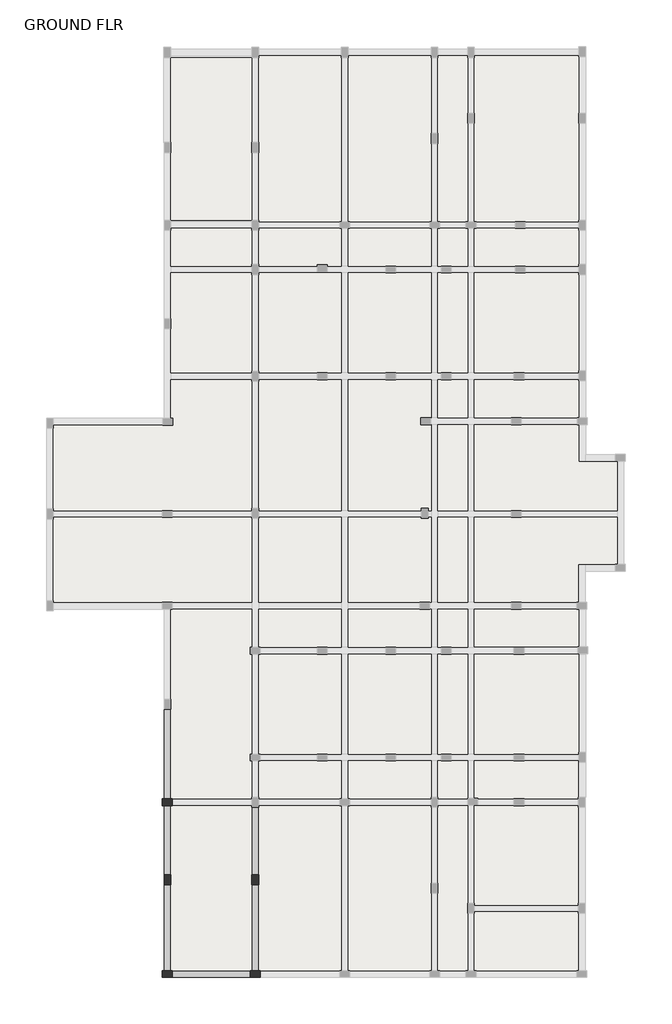
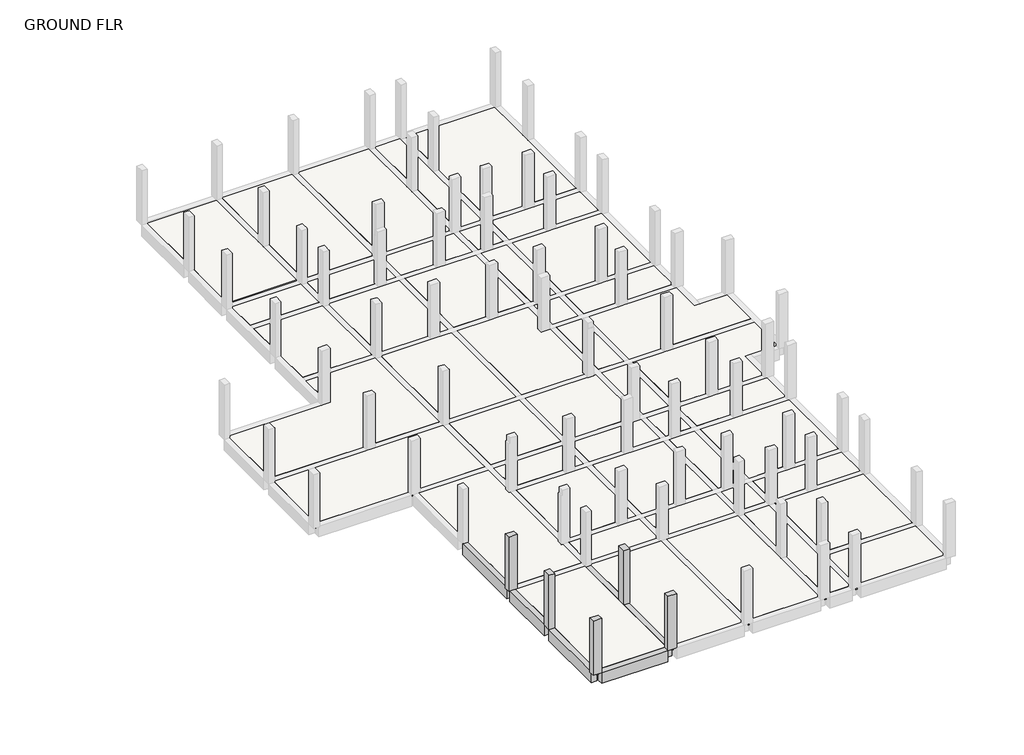
# One storey, part 1 of 5: 6 beams, 5 columns, 2 slabs.
"""IFC4 building model written with IfcOpenShell, lengths in millimetres."""

from ifc_helpers import new_model, si_unit, frame, origin, place, context, project, spatial, polyline, outline, extrude, faceted_brep, element, save

model = new_model("IFC4")

# Units and contexts
model_context = context("Model", 3, world=origin())
ifc_project = project(units=[si_unit("LENGTHUNIT", "METRE", prefix="MILLI")], contexts=[model_context])

# Site, building, storey
site = spatial("IfcSite", under=ifc_project)
building = spatial("IfcBuilding", under=site)
storey = spatial("IfcBuildingStorey", under=building, Name="GROUND FLR", Elevation=0.0)

# Beams
placement = place(None, origin())
element("IfcBeam", 1, ObjectType="M_Concrete-Rectangular Beam : 300 x 600mm", at=placement, inside=storey, context=model_context, shape_type="Brep", body=[
    faceted_brep([(-5588.8105653, -11607.8970059, 0.0), (-5588.8105653, -7619.0760584, 0.0), (-5888.8105653, -7619.0760584, 0.0), (-5888.8105653, -11607.8970059, 0.0), (-5888.8105653, -7619.0760584, -600.0), (-5888.8105653, -11607.8970059, -600.0), (-5588.8105653, -7619.0760584, -600.0), (-5588.8105653, -11607.8970059, -600.0), (-5588.8105653, -11607.8970059, -300.0), (-5588.8105653, -7619.0760584, -300.0)], [[[0, 1, 2, 3]], [[3, 2, 4, 5]], [[5, 4, 6, 7]], [[1, 0, 8, 7, 6, 9]], [[0, 3, 5, 7, 8]], [[6, 4, 2, 1, 9]]]),
])
element("IfcBeam", 2, ObjectType="M_Concrete-Rectangular Beam : 300 x 600mm", at=placement, inside=storey, context=model_context, shape_type="Brep", body=[
    faceted_brep([(-5588.8105653, -14991.2517597, 0.0), (-5588.8105653, -11907.8970059, 0.0), (-5888.8105653, -11907.8970059, 0.0), (-5888.8105653, -14991.2517597, 0.0), (-5888.8105653, -11907.8970059, -600.0), (-5888.8105653, -14991.2517597, -600.0), (-5588.8105653, -11907.8970059, -600.0), (-5588.8105653, -14991.2517597, -600.0), (-5588.8105653, -14991.2517597, -300.0), (-5588.8105653, -11907.8970059, -300.0)], [[[0, 1, 2, 3]], [[3, 2, 4, 5]], [[5, 4, 6, 7]], [[1, 0, 8, 7, 6, 9]], [[6, 4, 2, 1, 9]], [[0, 3, 5, 7, 8]]]),
])
element("IfcBeam", 3, ObjectType="M_Concrete-Rectangular Beam : 300 x 600mm", at=placement, inside=storey, context=model_context, shape_type="Brep", body=[
    faceted_brep([(-5588.8105653, -15441.2517597, 0.0), (-5888.8105653, -15441.2517597, 0.0), (-5888.8105653, -19272.5304373, 0.0), (-5588.8105653, -19272.5304373, 0.0), (-5888.8105653, -15441.2517597, -600.0), (-5888.8105653, -19272.5304373, -600.0), (-5588.8105653, -15441.2517597, -600.0), (-5588.8105653, -19272.5304373, -600.0), (-5588.8105653, -19272.5304373, -300.0), (-5588.8105653, -15441.2517597, -300.0)], [[[0, 1, 2, 3]], [[1, 4, 5, 2]], [[4, 6, 7, 5]], [[0, 3, 8, 7, 6, 9]], [[6, 4, 1, 0, 9]], [[3, 2, 5, 7, 8]]]),
])
element("IfcBeam", 4, ObjectType="M_Concrete-Rectangular Beam : 300 x 600mm", at=placement, inside=storey, context=model_context, shape_type="SweptSolid", body=[
    extrude(outline(polyline([(-2046.7865686, -19272.5304373), (-2046.7865686, -19572.5304373), (-5516.7865686, -19572.5304373), (-5516.7865686, -19272.5304373), (-2046.7865686, -19272.5304373)])), frame((0.0, 0.0, -600.0), z_axis=(0.0, 0.0, 1.0), x_axis=(1.0, 0.0, 0.0)), (0.0, 0.0, 1.0), 600.0),
])
element("IfcBeam", 5, ObjectType="M_Concrete-Rectangular Beam : 300 x 600mm", at=placement, inside=storey, context=model_context, shape_type="Brep", body=[
    faceted_brep([(-1971.7865686, -15441.2517597, 0.0), (-1971.7865686, -19272.5304373, 0.0), (-1671.7865686, -19272.5304373, 0.0), (-1671.7865686, -15441.2517597, 0.0), (-1671.7865686, -19272.5304373, -300.0), (-1671.7865686, -19272.5304373, -600.0), (-1671.7865686, -15441.2517597, -600.0), (-1671.7865686, -15441.2517597, -300.0), (-1971.7865686, -19272.5304373, -600.0), (-1971.7865686, -15441.2517597, -600.0), (-1971.7865686, -15441.2517597, -300.0), (-1971.7865686, -19272.5304373, -300.0)], [[[0, 1, 2, 3]], [[3, 2, 4, 5, 6, 7]], [[6, 5, 8, 9]], [[1, 0, 10, 9, 8, 11]], [[0, 3, 7, 6, 9, 10]], [[8, 5, 4, 2, 1, 11]]]),
])
element("IfcBeam", 6, ObjectType="M_Concrete-Rectangular Beam : 300 x 600mm", at=placement, inside=storey, context=model_context, shape_type="Brep", body=[
    faceted_brep([(-1971.7865686, -11982.8970059, 0.0), (-1971.7865686, -14991.2517597, 0.0), (-1671.7865686, -14991.2517597, 0.0), (-1671.7865686, -11982.8970059, 0.0), (-1671.7865686, -14991.2517597, -300.0), (-1671.7865686, -14991.2517597, -600.0), (-1671.7865686, -11982.8970059, -600.0), (-1671.7865686, -11982.8970059, -300.0), (-1971.7865686, -14991.2517597, -600.0), (-1971.7865686, -11982.8970059, -600.0), (-1971.7865686, -11982.8970059, -300.0), (-1971.7865686, -14991.2517597, -300.0)], [[[0, 1, 2, 3]], [[3, 2, 4, 5, 6, 7]], [[6, 5, 8, 9]], [[1, 0, 10, 9, 8, 11]], [[0, 3, 7, 6, 9, 10]], [[8, 5, 4, 2, 1, 11]]]),
])

# Columns
element("IfcColumn", 7, ObjectType="M_Concrete-Rectangular-Column : 300 x 450mm", at=placement, inside=storey, context=model_context, shape_type="Brep", body=[
    faceted_brep([(-5513.8105653, -11907.8970059, 0.0), (-5963.8105653, -11907.8970059, 0.0), (-5963.8105653, -11607.8970059, 0.0), (-5513.8105653, -11607.8970059, 0.0), (-5513.8105653, -11907.8970059, 2700.0), (-5513.8105653, -11907.8970059, 3000.0), (-5588.8105653, -11907.8970059, 3000.0), (-5963.8105653, -11907.8970059, 3000.0), (-5963.8105653, -11607.8970059, 3000.0), (-5588.8105653, -11607.8970059, 3000.0), (-5513.8105653, -11607.8970059, 3000.0), (-5513.8105653, -11607.8970059, 2700.0)], [[[0, 1, 2, 3]], [[1, 0, 4, 5, 6, 7]], [[2, 1, 7, 8]], [[3, 2, 8, 9, 10, 11]], [[0, 3, 11, 10, 5, 4]], [[8, 7, 6, 5, 10, 9]]]),
])
element("IfcColumn", 8, ObjectType="M_Concrete-Rectangular-Column : 300 x 450mm", at=placement, inside=storey, context=model_context, shape_type="Brep", body=[
    faceted_brep([(-5588.8105653, -14991.2517597, 0.0), (-5588.8105653, -15441.2517597, 0.0), (-5888.8105653, -15441.2517597, 0.0), (-5888.8105653, -14991.2517597, 0.0), (-5588.8105653, -14991.2517597, 2700.0), (-5588.8105653, -14991.2517597, 3000.0), (-5588.8105653, -15441.2517597, 3000.0), (-5588.8105653, -15441.2517597, 2700.0), (-5888.8105653, -15441.2517597, 3000.0), (-5888.8105653, -14991.2517597, 3000.0)], [[[0, 1, 2, 3]], [[1, 0, 4, 5, 6, 7]], [[2, 1, 7, 6, 8]], [[3, 2, 8, 9]], [[0, 3, 9, 5, 4]], [[6, 5, 9, 8]]]),
])
element("IfcColumn", 9, ObjectType="M_Concrete-Rectangular-Column : 300 x 450mm", at=placement, inside=storey, context=model_context, shape_type="Brep", body=[
    faceted_brep([(-1671.7865686, -14991.2517597, 0.0), (-1671.7865686, -15441.2517597, 0.0), (-1971.7865686, -15441.2517597, 0.0), (-1971.7865686, -14991.2517597, 0.0), (-1671.7865686, -14991.2517597, 2700.0), (-1671.7865686, -14991.2517597, 3000.0), (-1671.7865686, -15441.2517597, 3000.0), (-1671.7865686, -15441.2517597, 2700.0), (-1971.7865686, -15441.2517597, 3000.0), (-1971.7865686, -15441.2517597, 2700.0), (-1971.7865686, -14991.2517597, 3000.0), (-1971.7865686, -14991.2517597, 2700.0)], [[[0, 1, 2, 3]], [[1, 0, 4, 5, 6, 7]], [[2, 1, 7, 6, 8, 9]], [[3, 2, 9, 8, 10, 11]], [[0, 3, 11, 10, 5, 4]], [[6, 5, 10, 8]]]),
])
element("IfcColumn", 10, ObjectType="M_Concrete-Rectangular-Column : 300 x 450mm", at=placement, inside=storey, context=model_context, shape_type="Brep", body=[
    faceted_brep([(-2046.7865686, -19272.5304373, 0.0), (-1596.7865686, -19272.5304373, 0.0), (-1596.7865686, -19572.5304373, 0.0), (-2046.7865686, -19572.5304373, 0.0), (-2046.7865686, -19272.5304373, 3000.0), (-1971.7865686, -19272.5304373, 3000.0), (-1671.7865686, -19272.5304373, 3000.0), (-1596.7865686, -19272.5304373, 3000.0), (-1596.7865686, -19572.5304373, 3000.0), (-2046.7865686, -19572.5304373, 3000.0)], [[[0, 1, 2, 3]], [[4, 5, 6, 7, 1, 0]], [[7, 8, 2, 1]], [[8, 9, 3, 2]], [[9, 4, 0, 3]], [[4, 9, 8, 7, 6, 5]]]),
])
element("IfcColumn", 11, ObjectType="M_Concrete-Rectangular-Column : 300 x 450mm", at=placement, inside=storey, context=model_context, shape_type="Brep", body=[
    faceted_brep([(-5516.7865686, -19572.5304373, 0.0), (-5966.7865686, -19572.5304373, 0.0), (-5966.7865686, -19272.5304373, 0.0), (-5516.7865686, -19272.5304373, 0.0), (-5516.7865686, -19572.5304373, 3000.0), (-5966.7865686, -19572.5304373, 3000.0), (-5966.7865686, -19272.5304373, 3000.0), (-5588.8105653, -19272.5304373, 3000.0), (-5516.7865686, -19272.5304373, 3000.0)], [[[0, 1, 2, 3]], [[4, 5, 1, 0]], [[5, 6, 2, 1]], [[6, 7, 8, 3, 2]], [[8, 4, 0, 3]], [[4, 8, 7, 6, 5]]]),
])

# Slabs
element("IfcSlab", 12, ObjectType="Generic 300mm", at=placement, inside=storey, context=model_context, shape_type="Brep", body=[
    faceted_brep([(-1971.7865686, 21462.8349362, -300.0), (-1971.7865686, 14212.5179708, -300.0), (-5588.8105653, 14212.5179708, -300.0), (-5591.7865686, 14212.5179708, -300.0), (-5591.7865686, 17224.7148651, -300.0), (-5591.7865686, 17674.7148651, -300.0), (-5591.7865686, 21462.8349362, -300.0), (-1971.7865686, 21462.8349362, 0.0), (-5591.7865686, 21462.8349362, 0.0), (-5591.7865686, 17674.7148651, 0.0), (-5591.7865686, 17224.7148651, 0.0), (-5591.7865686, 14212.5179708, 0.0), (-5588.8105653, 14212.5179708, 0.0), (-1971.7865686, 14212.5179708, 0.0), (-1971.7865686, 17224.7148651, 0.0), (-1971.7865686, 17674.7148651, 0.0)], [[[0, 1, 2, 3, 4, 5, 6]], [[7, 8, 9, 10, 11, 12, 13, 14, 15]], [[1, 0, 7, 15, 14, 13]], [[3, 2, 1, 13, 12, 11]], [[6, 5, 4, 3, 11, 10, 9, 8]], [[0, 6, 8, 7]]]),
    faceted_brep([(2024.7296816, 21537.8349362, -300.0), (2024.7296816, 14137.5179708, -300.0), (-1671.7865686, 14137.5179708, -300.0), (-1671.7865686, 21537.8349362, -300.0), (2024.7296816, 21537.8349362, 0.0), (-1671.7865686, 21537.8349362, 0.0), (-1671.7865686, 21462.8349362, 0.0), (-1671.7865686, 17674.7148651, 0.0), (-1671.7865686, 17224.7148651, 0.0), (-1671.7865686, 14212.5179708, 0.0), (-1671.7865686, 14137.5179708, 0.0), (1949.7296816, 14137.5179708, 0.0), (2024.7296816, 14137.5179708, 0.0), (2024.7296816, 21462.8349362, 0.0)], [[[0, 1, 2, 3]], [[4, 5, 6, 7, 8, 9, 10, 11, 12, 13]], [[1, 0, 4, 13, 12]], [[2, 1, 12, 11, 10]], [[3, 2, 10, 9, 8, 7, 6, 5]], [[0, 3, 5, 4]]]),
    faceted_brep([(6032.5248054, 21537.8349362, -300.0), (6032.5248054, 14137.5179708, -300.0), (2324.7296816, 14137.5179708, -300.0), (2324.7296816, 21537.8349362, -300.0), (6032.5248054, 21537.8349362, 0.0), (2324.7296816, 21537.8349362, 0.0), (2324.7296816, 21462.8349362, 0.0), (2324.7296816, 14137.5179708, 0.0), (2399.7296816, 14137.5179708, 0.0), (5957.5248054, 14137.5179708, 0.0), (6032.5248054, 14137.5179708, 0.0), (6032.5248054, 17624.7148651, 0.0), (6032.5248054, 18074.7148651, 0.0), (6032.5248054, 21462.8349362, 0.0)], [[[0, 1, 2, 3]], [[4, 5, 6, 7, 8, 9, 10, 11, 12, 13]], [[1, 0, 4, 13, 12, 11, 10]], [[2, 1, 10, 9, 8, 7]], [[3, 2, 7, 6, 5]], [[0, 3, 5, 4]]]),
    faceted_brep([(7656.8679014, 21537.8349362, -300.0), (7656.8679014, 14137.5179708, -300.0), (6332.5248054, 14137.5179708, -300.0), (6332.5248054, 21537.8349362, -300.0), (7656.8679014, 21537.8349362, 0.0), (6332.5248054, 21537.8349362, 0.0), (6332.5248054, 21462.8349362, 0.0), (6332.5248054, 18074.7148651, 0.0), (6332.5248054, 17624.7148651, 0.0), (6332.5248054, 14137.5179708, 0.0), (6407.5248054, 14137.5179708, 0.0), (7581.8679014, 14137.5179708, 0.0), (7656.8679014, 14137.5179708, 0.0), (7656.8679014, 18524.7148651, 0.0), (7656.8679014, 18974.7148651, 0.0), (7656.8679014, 21462.8349362, 0.0)], [[[0, 1, 2, 3]], [[4, 5, 6, 7, 8, 9, 10, 11, 12, 13, 14, 15]], [[1, 0, 4, 15, 14, 13, 12]], [[2, 1, 12, 11, 10, 9]], [[3, 2, 9, 8, 7, 6, 5]], [[0, 3, 5, 4]]]),
    faceted_brep([(12619.1163908, 21537.8349362, -300.0), (12619.1163908, 14137.5179708, -300.0), (7956.8679014, 14137.5179708, -300.0), (7956.8679014, 21537.8349362, -300.0), (12619.1163908, 21537.8349362, 0.0), (7956.8679014, 21537.8349362, 0.0), (7956.8679014, 21462.8349362, 0.0), (7956.8679014, 18974.7148651, 0.0), (7956.8679014, 18524.7148651, 0.0), (7956.8679014, 14137.5179708, 0.0), (8031.8679014, 14137.5179708, 0.0), (9781.8679014, 14137.5179708, 0.0), (10231.8679014, 14137.5179708, 0.0), (12619.1163908, 14137.5179708, 0.0), (12619.1163908, 14212.5179708, 0.0), (12619.1163908, 18524.7148651, 0.0), (12619.1163908, 18974.7148651, 0.0), (12619.1163908, 21502.8349362, 0.0)], [[[0, 1, 2, 3]], [[4, 5, 6, 7, 8, 9, 10, 11, 12, 13, 14, 15, 16, 17]], [[1, 0, 4, 17, 16, 15, 14, 13]], [[2, 1, 13, 12, 11, 10, 9]], [[3, 2, 9, 8, 7, 6, 5]], [[0, 3, 5, 4]]]),
    faceted_brep([(-1971.7865686, 13837.5179708, -300.0), (-1971.7865686, 12157.4075451, -300.0), (-5588.8105653, 12157.4075451, -300.0), (-5588.8105653, 13837.5179708, -300.0), (-1971.7865686, 13837.5179708, 0.0), (-5588.8105653, 13837.5179708, 0.0), (-5588.8105653, 13762.5179708, 0.0), (-5588.8105653, 12157.4075451, 0.0), (-1971.7865686, 12157.4075451, 0.0), (-1971.7865686, 12232.4075451, 0.0), (-1971.7865686, 13762.5179708, 0.0)], [[[0, 1, 2, 3]], [[4, 5, 6, 7, 8, 9, 10]], [[1, 0, 4, 10, 9, 8]], [[2, 1, 8, 7]], [[3, 2, 7, 6, 5]], [[0, 3, 5, 4]]]),
    faceted_brep([(2024.7296816, 13837.5179708, -300.0), (2024.7296816, 12157.4075451, -300.0), (1399.7296816, 12157.4075451, -300.0), (949.7296816, 12157.4075451, -300.0), (-1671.7865686, 12157.4075451, -300.0), (-1671.7865686, 13837.5179708, -300.0), (2024.7296816, 13837.5179708, 0.0), (1949.7296816, 13837.5179708, 0.0), (-1671.7865686, 13837.5179708, 0.0), (-1671.7865686, 13762.5179708, 0.0), (-1671.7865686, 12232.4075451, 0.0), (-1671.7865686, 12157.4075451, 0.0), (949.7296816, 12157.4075451, 0.0), (1399.7296816, 12157.4075451, 0.0), (2024.7296816, 12157.4075451, 0.0)], [[[0, 1, 2, 3, 4, 5]], [[6, 7, 8, 9, 10, 11, 12, 13, 14]], [[1, 0, 6, 14]], [[4, 3, 2, 1, 14, 13, 12, 11]], [[5, 4, 11, 10, 9, 8]], [[0, 5, 8, 7, 6]]]),
    faceted_brep([(6032.5248054, 13837.5179708, -300.0), (6032.5248054, 12157.4075451, -300.0), (2324.7296816, 12157.4075451, -300.0), (2324.7296816, 13837.5179708, -300.0), (6032.5248054, 13837.5179708, 0.0), (5957.5248054, 13837.5179708, 0.0), (2399.7296816, 13837.5179708, 0.0), (2324.7296816, 13837.5179708, 0.0), (2324.7296816, 12157.4075451, 0.0), (3997.5248054, 12157.4075451, 0.0), (4447.5248054, 12157.4075451, 0.0), (6032.5248054, 12157.4075451, 0.0)], [[[0, 1, 2, 3]], [[4, 5, 6, 7, 8, 9, 10, 11]], [[1, 0, 4, 11]], [[2, 1, 11, 10, 9, 8]], [[3, 2, 8, 7]], [[0, 3, 7, 6, 5, 4]]]),
    faceted_brep([(7656.8679014, 13837.5179708, -300.0), (7656.8679014, 12157.4075451, -300.0), (6332.5248054, 12157.4075451, -300.0), (6332.5248054, 13837.5179708, -300.0), (7656.8679014, 13837.5179708, 0.0), (7581.8679014, 13837.5179708, 0.0), (6407.5248054, 13837.5179708, 0.0), (6332.5248054, 13837.5179708, 0.0), (6332.5248054, 12157.4075451, 0.0), (6481.8679014, 12157.4075451, 0.0), (6931.8679014, 12157.4075451, 0.0), (7656.8679014, 12157.4075451, 0.0)], [[[0, 1, 2, 3]], [[4, 5, 6, 7, 8, 9, 10, 11]], [[1, 0, 4, 11]], [[2, 1, 11, 10, 9, 8]], [[3, 2, 8, 7]], [[0, 3, 7, 6, 5, 4]]]),
    faceted_brep([(12619.1163908, 13837.5179708, -300.0), (12619.1163908, 12157.4075451, -300.0), (7956.8679014, 12157.4075451, -300.0), (7956.8679014, 13837.5179708, -300.0), (12619.1163908, 13837.5179708, 0.0), (10231.8679014, 13837.5179708, 0.0), (9781.8679014, 13837.5179708, 0.0), (8031.8679014, 13837.5179708, 0.0), (7956.8679014, 13837.5179708, 0.0), (7956.8679014, 12157.4075451, 0.0), (9781.8679014, 12157.4075451, 0.0), (10231.8679014, 12157.4075451, 0.0), (12619.1163908, 12157.4075451, 0.0), (12619.1163908, 12232.4075451, 0.0), (12619.1163908, 13762.5179708, 0.0)], [[[0, 1, 2, 3]], [[4, 5, 6, 7, 8, 9, 10, 11, 12, 13, 14]], [[1, 0, 4, 14, 13, 12]], [[2, 1, 12, 11, 10, 9]], [[3, 2, 9, 8]], [[0, 3, 8, 7, 6, 5, 4]]]),
    faceted_brep([(-1971.7865686, 11857.4075451, -300.0), (-1971.7865686, 7399.7076276, -300.0), (-5588.8105653, 7399.7076276, -300.0), (-5588.8105653, 11857.4075451, -300.0), (-1971.7865686, 11857.4075451, 0.0), (-5588.8105653, 11857.4075451, 0.0), (-5588.8105653, 9817.5252033, 0.0), (-5588.8105653, 9367.5252033, 0.0), (-5588.8105653, 7399.7076276, 0.0), (-1971.7865686, 7399.7076276, 0.0), (-1971.7865686, 7474.7076276, 0.0), (-1971.7865686, 11782.4075451, 0.0)], [[[0, 1, 2, 3]], [[4, 5, 6, 7, 8, 9, 10, 11]], [[1, 0, 4, 11, 10, 9]], [[2, 1, 9, 8]], [[3, 2, 8, 7, 6, 5]], [[0, 3, 5, 4]]]),
    faceted_brep([(2024.7296816, 11857.4075451, -300.0), (2024.7296816, 7399.7076276, -300.0), (-1671.7865686, 7399.7076276, -300.0), (-1671.7865686, 11857.4075451, -300.0), (2024.7296816, 11857.4075451, 0.0), (-1671.7865686, 11857.4075451, 0.0), (-1671.7865686, 11782.4075451, 0.0), (-1671.7865686, 7474.7076276, 0.0), (-1671.7865686, 7399.7076276, 0.0), (949.7296816, 7399.7076276, 0.0), (1399.7296816, 7399.7076276, 0.0), (2024.7296816, 7399.7076276, 0.0)], [[[0, 1, 2, 3]], [[4, 5, 6, 7, 8, 9, 10, 11]], [[1, 0, 4, 11]], [[2, 1, 11, 10, 9, 8]], [[3, 2, 8, 7, 6, 5]], [[0, 3, 5, 4]]]),
    faceted_brep([(6032.5248054, 11857.4075451, -300.0), (6032.5248054, 7399.7076276, -300.0), (2324.7296816, 7399.7076276, -300.0), (2324.7296816, 11857.4075451, -300.0), (6032.5248054, 11857.4075451, 0.0), (4447.5248054, 11857.4075451, 0.0), (3997.5248054, 11857.4075451, 0.0), (2324.7296816, 11857.4075451, 0.0), (2324.7296816, 7399.7076276, 0.0), (3997.5248054, 7399.7076276, 0.0), (4447.5248054, 7399.7076276, 0.0), (6032.5248054, 7399.7076276, 0.0)], [[[0, 1, 2, 3]], [[4, 5, 6, 7, 8, 9, 10, 11]], [[1, 0, 4, 11]], [[2, 1, 11, 10, 9, 8]], [[3, 2, 8, 7]], [[0, 3, 7, 6, 5, 4]]]),
    faceted_brep([(7656.8679014, 11857.4075451, -300.0), (7656.8679014, 7399.7076276, -300.0), (6332.5248054, 7399.7076276, -300.0), (6332.5248054, 11857.4075451, -300.0), (7656.8679014, 11857.4075451, 0.0), (6931.8679014, 11857.4075451, 0.0), (6481.8679014, 11857.4075451, 0.0), (6332.5248054, 11857.4075451, 0.0), (6332.5248054, 7399.7076276, 0.0), (6481.8679014, 7399.7076276, 0.0), (6931.8679014, 7399.7076276, 0.0), (7656.8679014, 7399.7076276, 0.0)], [[[0, 1, 2, 3]], [[4, 5, 6, 7, 8, 9, 10, 11]], [[1, 0, 4, 11]], [[2, 1, 11, 10, 9, 8]], [[3, 2, 8, 7]], [[0, 3, 7, 6, 5, 4]]]),
    faceted_brep([(12616.8679014, 11857.4075451, -300.0), (12616.8679014, 7399.7076276, -300.0), (7956.8679014, 7399.7076276, -300.0), (7956.8679014, 11857.4075451, -300.0), (12616.8679014, 11857.4075451, 0.0), (10231.8679014, 11857.4075451, 0.0), (9781.8679014, 11857.4075451, 0.0), (7956.8679014, 11857.4075451, 0.0), (7956.8679014, 7399.7076276, 0.0), (9721.8679014, 7399.7076276, 0.0), (10171.8679014, 7399.7076276, 0.0), (12616.8679014, 7399.7076276, 0.0)], [[[0, 1, 2, 3]], [[4, 5, 6, 7, 8, 9, 10, 11]], [[1, 0, 4, 11]], [[2, 1, 11, 10, 9, 8]], [[3, 2, 8, 7]], [[0, 3, 7, 6, 5, 4]]]),
    faceted_brep([(7656.8679014, 7099.7076276, -300.0), (7656.8679014, 5387.6057249, -300.0), (6332.5248054, 5387.6057249, -300.0), (6332.5248054, 7099.7076276, -300.0), (7656.8679014, 7099.7076276, 0.0), (6931.8679014, 7099.7076276, 0.0), (6481.8679014, 7099.7076276, 0.0), (6332.5248054, 7099.7076276, 0.0), (6332.5248054, 5387.6057249, 0.0), (7656.8679014, 5387.6057249, 0.0)], [[[0, 1, 2, 3]], [[4, 5, 6, 7, 8, 9]], [[1, 0, 4, 9]], [[2, 1, 9, 8]], [[3, 2, 8, 7]], [[0, 3, 7, 6, 5, 4]]]),
    faceted_brep([(12616.8679014, 7099.7076276, -300.0), (12616.8679014, 5387.6057249, -300.0), (7956.8679014, 5387.6057249, -300.0), (7956.8679014, 7099.7076276, -300.0), (12616.8679014, 7099.7076276, 0.0), (10171.8679014, 7099.7076276, 0.0), (9721.8679014, 7099.7076276, 0.0), (7956.8679014, 7099.7076276, 0.0), (7956.8679014, 5387.6057249, 0.0), (9601.8679014, 5387.6057249, 0.0), (10051.8679014, 5387.6057249, 0.0), (12541.8679014, 5387.6057249, 0.0), (12616.8679014, 5387.6057249, 0.0)], [[[0, 1, 2, 3]], [[4, 5, 6, 7, 8, 9, 10, 11, 12]], [[1, 0, 4, 12]], [[2, 1, 12, 11, 10, 9, 8]], [[3, 2, 8, 7]], [[0, 3, 7, 6, 5, 4]]]),
    faceted_brep([(7656.8679014, 5087.6057249, -300.0), (7656.8679014, 1251.1713929, -300.0), (6332.5248054, 1251.1713929, -300.0), (6332.5248054, 5087.6057249, -300.0), (7656.8679014, 5087.6057249, 0.0), (6332.5248054, 5087.6057249, 0.0), (6332.5248054, 1251.1713929, 0.0), (7656.8679014, 1251.1713929, 0.0)], [[[0, 1, 2, 3]], [[4, 5, 6, 7]], [[1, 0, 4, 7]], [[2, 1, 7, 6]], [[3, 2, 6, 5]], [[0, 3, 5, 4]]]),
    faceted_brep([(14319.1163908, 1251.1713929, -300.0), (7956.8679014, 1251.1713929, -300.0), (7956.8679014, 5087.6057249, -300.0), (12616.8679014, 5087.6057249, -300.0), (12616.8679014, 3435.7536525, -300.0), (14319.1163908, 3435.7536525, -300.0), (14319.1163908, 1251.1713929, 0.0), (14319.1163908, 3435.7536525, 0.0), (12916.8679014, 3435.7536525, 0.0), (12616.8679014, 3435.7536525, 0.0), (12616.8679014, 5087.6057249, 0.0), (12541.8679014, 5087.6057249, 0.0), (10051.8679014, 5087.6057249, 0.0), (9601.8679014, 5087.6057249, 0.0), (7956.8679014, 5087.6057249, 0.0), (7956.8679014, 1251.1713929, 0.0), (9601.8679014, 1251.1713929, 0.0), (10051.8679014, 1251.1713929, 0.0)], [[[0, 1, 2, 3, 4, 5]], [[6, 7, 8, 9, 10, 11, 12, 13, 14, 15, 16, 17]], [[1, 0, 6, 17, 16, 15]], [[2, 1, 15, 14]], [[3, 2, 14, 13, 12, 11, 10]], [[4, 3, 10, 9]], [[5, 4, 9, 8, 7]], [[0, 5, 7, 6]]]),
    faceted_brep([(7956.8679014, -2839.4535766, -300.0), (7956.8679014, 951.1713929, -300.0), (14319.1163908, 951.1713929, -300.0), (14319.1163908, -1148.8286071, -300.0), (12599.1163908, -1148.8286071, -300.0), (12599.1163908, -2839.4535766, -300.0), (7956.8679014, -2839.4535766, 0.0), (9601.8679014, -2839.4535766, 0.0), (10051.8679014, -2839.4535766, 0.0), (12524.1163908, -2839.4535766, 0.0), (12599.1163908, -2839.4535766, 0.0), (12599.1163908, -1148.8286071, 0.0), (12899.1163908, -1148.8286071, 0.0), (14244.1163908, -1148.8286071, 0.0), (14319.1163908, -1148.8286071, 0.0), (14319.1163908, 951.1713929, 0.0), (10051.8679014, 951.1713929, 0.0), (9601.8679014, 951.1713929, 0.0), (7956.8679014, 951.1713929, 0.0)], [[[0, 1, 2, 3, 4, 5]], [[6, 7, 8, 9, 10, 11, 12, 13, 14, 15, 16, 17, 18]], [[1, 0, 6, 18]], [[2, 1, 18, 17, 16, 15]], [[3, 2, 15, 14]], [[4, 3, 14, 13, 12, 11]], [[5, 4, 11, 10]], [[0, 5, 10, 9, 8, 7, 6]]]),
    faceted_brep([(7656.8679014, 951.1713929, -300.0), (7656.8679014, -2839.4535766, -300.0), (6332.5248054, -2839.4535766, -300.0), (6332.5248054, 951.1713929, -300.0), (7656.8679014, 951.1713929, 0.0), (6332.5248054, 951.1713929, 0.0), (6332.5248054, -2839.4535766, 0.0), (7656.8679014, -2839.4535766, 0.0)], [[[0, 1, 2, 3]], [[4, 5, 6, 7]], [[1, 0, 4, 7]], [[2, 1, 7, 6]], [[3, 2, 6, 5]], [[0, 3, 5, 4]]]),
    faceted_brep([(6032.5248054, 951.1713929, -300.0), (6032.5248054, -2839.4535766, -300.0), (2324.7296816, -2839.4535766, -300.0), (2324.7296816, 951.1713929, -300.0), (5592.5248054, 951.1713929, -300.0), (5892.5248054, 951.1713929, -300.0), (6032.5248054, 951.1713929, 0.0), (5892.5248054, 951.1713929, 0.0), (5592.5248054, 951.1713929, 0.0), (2324.7296816, 951.1713929, 0.0), (2324.7296816, -2839.4535766, 0.0), (5517.5248054, -2839.4535766, 0.0), (5967.5248054, -2839.4535766, 0.0), (6032.5248054, -2839.4535766, 0.0)], [[[0, 1, 2, 3, 4, 5]], [[6, 7, 8, 9, 10, 11, 12, 13]], [[1, 0, 6, 13]], [[2, 1, 13, 12, 11, 10]], [[3, 2, 10, 9]], [[0, 5, 4, 3, 9, 8, 7, 6]]]),
    faceted_brep([(2024.7296816, 951.1713929, -300.0), (2024.7296816, -2839.4535766, -300.0), (-1671.7865686, -2839.4535766, -300.0), (-1671.7865686, 951.1713929, -300.0), (2024.7296816, 951.1713929, 0.0), (-1671.7865686, 951.1713929, 0.0), (-1671.7865686, 916.1713929, 0.0), (-1671.7865686, -2839.4535766, 0.0), (2024.7296816, -2839.4535766, 0.0)], [[[0, 1, 2, 3]], [[4, 5, 6, 7, 8]], [[1, 0, 4, 8]], [[2, 1, 8, 7]], [[3, 2, 7, 6, 5]], [[0, 3, 5, 4]]]),
    faceted_brep([(2024.7296816, 7099.7076276, -300.0), (2024.7296816, 1251.1713929, -300.0), (-1671.7865686, 1251.1713929, -300.0), (-1671.7865686, 7099.7076276, -300.0), (2024.7296816, 7099.7076276, 0.0), (1399.7296816, 7099.7076276, 0.0), (949.7296816, 7099.7076276, 0.0), (-1671.7865686, 7099.7076276, 0.0), (-1671.7865686, 7024.7076276, 0.0), (-1671.7865686, 1366.1713929, 0.0), (-1671.7865686, 1251.1713929, 0.0), (2024.7296816, 1251.1713929, 0.0)], [[[0, 1, 2, 3]], [[4, 5, 6, 7, 8, 9, 10, 11]], [[1, 0, 4, 11]], [[2, 1, 11, 10]], [[3, 2, 10, 9, 8, 7]], [[0, 3, 7, 6, 5, 4]]]),
    faceted_brep([(-10828.8105653, 1251.1713929, -300.0), (-10828.8105653, 5067.6057249, -300.0), (-5493.8105653, 5067.6057249, -300.0), (-5493.8105653, 5367.5252033, -300.0), (-5588.8105653, 5367.5252033, -300.0), (-5588.8105653, 7099.7076276, -300.0), (-1971.7865686, 7099.7076276, -300.0), (-1971.7865686, 1251.1713929, -300.0), (-10828.8105653, 1251.1713929, 0.0), (-5963.8105653, 1251.1713929, 0.0), (-5513.8105653, 1251.1713929, 0.0), (-1971.7865686, 1251.1713929, 0.0), (-1971.7865686, 1366.1713929, 0.0), (-1971.7865686, 7024.7076276, 0.0), (-1971.7865686, 7099.7076276, 0.0), (-5588.8105653, 7099.7076276, 0.0), (-5588.8105653, 5367.5252033, 0.0), (-5493.8105653, 5367.5252033, 0.0), (-5493.8105653, 5067.6057249, 0.0), (-5943.8105653, 5067.6057249, 0.0), (-10828.8105653, 5067.6057249, 0.0), (-10828.8105653, 4932.6057249, 0.0), (-10828.8105653, 1326.1713929, 0.0)], [[[0, 1, 2, 3, 4, 5, 6, 7]], [[8, 9, 10, 11, 12, 13, 14, 15, 16, 17, 18, 19, 20, 21, 22]], [[1, 0, 8, 22, 21, 20]], [[2, 1, 20, 19, 18]], [[3, 2, 18, 17]], [[4, 3, 17, 16]], [[5, 4, 16, 15]], [[6, 5, 15, 14]], [[7, 6, 14, 13, 12, 11]], [[0, 7, 11, 10, 9, 8]]]),
    faceted_brep([(-1971.7865686, -2839.4535766, -300.0), (-10828.8105653, -2839.4535766, -300.0), (-10828.8105653, 951.1713929, -300.0), (-1971.7865686, 951.1713929, -300.0), (-1971.7865686, -2839.4535766, 0.0), (-1971.7865686, 916.1713929, 0.0), (-1971.7865686, 951.1713929, 0.0), (-5513.8105653, 951.1713929, 0.0), (-5963.8105653, 951.1713929, 0.0), (-10828.8105653, 951.1713929, 0.0), (-10828.8105653, 876.1713929, 0.0), (-10828.8105653, -2764.4535766, 0.0), (-10828.8105653, -2839.4535766, 0.0), (-5963.8105653, -2839.4535766, 0.0), (-5513.8105653, -2839.4535766, 0.0)], [[[0, 1, 2, 3]], [[4, 5, 6, 7, 8, 9, 10, 11, 12, 13, 14]], [[1, 0, 4, 14, 13, 12]], [[2, 1, 12, 11, 10, 9]], [[3, 2, 9, 8, 7, 6]], [[0, 3, 6, 5, 4]]]),
    faceted_brep([(2024.7296816, -3139.4535766, -300.0), (2024.7296816, -4851.6229916, -300.0), (-1671.7865686, -4851.6229916, -300.0), (-1671.7865686, -3139.4535766, -300.0), (2024.7296816, -3139.4535766, 0.0), (-1671.7865686, -3139.4535766, 0.0), (-1671.7865686, -4851.6229916, 0.0), (-1596.7865686, -4851.6229916, 0.0), (949.7296816, -4851.6229916, 0.0), (1399.7296816, -4851.6229916, 0.0), (2024.7296816, -4851.6229916, 0.0)], [[[0, 1, 2, 3]], [[4, 5, 6, 7, 8, 9, 10]], [[1, 0, 4, 10]], [[2, 1, 10, 9, 8, 7, 6]], [[3, 2, 6, 5]], [[0, 3, 5, 4]]]),
    faceted_brep([(6032.5248054, -3139.4535766, -300.0), (6032.5248054, -4851.6229916, -300.0), (2324.7296816, -4851.6229916, -300.0), (2324.7296816, -3139.4535766, -300.0), (6032.5248054, -3139.4535766, 0.0), (5967.5248054, -3139.4535766, 0.0), (5517.5248054, -3139.4535766, 0.0), (2324.7296816, -3139.4535766, 0.0), (2324.7296816, -4851.6229916, 0.0), (3997.5248054, -4851.6229916, 0.0), (4447.5248054, -4851.6229916, 0.0), (6032.5248054, -4851.6229916, 0.0)], [[[0, 1, 2, 3]], [[4, 5, 6, 7, 8, 9, 10, 11]], [[1, 0, 4, 11]], [[2, 1, 11, 10, 9, 8]], [[3, 2, 8, 7]], [[0, 3, 7, 6, 5, 4]]]),
    faceted_brep([(2024.7296816, -5151.6229916, -300.0), (2024.7296816, -9607.1078267, -300.0), (-1671.7865686, -9607.1078267, -300.0), (-1671.7865686, -5151.6229916, -300.0), (2024.7296816, -5151.6229916, 0.0), (1399.7296816, -5151.6229916, 0.0), (949.7296816, -5151.6229916, 0.0), (-1596.7865686, -5151.6229916, 0.0), (-1671.7865686, -5151.6229916, 0.0), (-1671.7865686, -9607.1078267, 0.0), (-1596.7865686, -9607.1078267, 0.0), (949.7296816, -9607.1078267, 0.0), (1399.7296816, -9607.1078267, 0.0), (2024.7296816, -9607.1078267, 0.0)], [[[0, 1, 2, 3]], [[4, 5, 6, 7, 8, 9, 10, 11, 12, 13]], [[1, 0, 4, 13]], [[2, 1, 13, 12, 11, 10, 9]], [[3, 2, 9, 8]], [[0, 3, 8, 7, 6, 5, 4]]]),
    faceted_brep([(6032.5248054, -5151.6229916, -300.0), (6032.5248054, -9607.1078267, -300.0), (2324.7296816, -9607.1078267, -300.0), (2324.7296816, -5151.6229916, -300.0), (6032.5248054, -5151.6229916, 0.0), (4447.5248054, -5151.6229916, 0.0), (3997.5248054, -5151.6229916, 0.0), (2324.7296816, -5151.6229916, 0.0), (2324.7296816, -9607.1078267, 0.0), (3997.5248054, -9607.1078267, 0.0), (4447.5248054, -9607.1078267, 0.0), (6032.5248054, -9607.1078267, 0.0)], [[[0, 1, 2, 3]], [[4, 5, 6, 7, 8, 9, 10, 11]], [[1, 0, 4, 11]], [[2, 1, 11, 10, 9, 8]], [[3, 2, 8, 7]], [[0, 3, 7, 6, 5, 4]]]),
    faceted_brep([(7656.8679014, -5151.6229916, -300.0), (7656.8679014, -9607.1078267, -300.0), (6332.5248054, -9607.1078267, -300.0), (6332.5248054, -5151.6229916, -300.0), (7656.8679014, -5151.6229916, 0.0), (6931.8679014, -5151.6229916, 0.0), (6481.8679014, -5151.6229916, 0.0), (6332.5248054, -5151.6229916, 0.0), (6332.5248054, -9607.1078267, 0.0), (6481.8679014, -9607.1078267, 0.0), (6931.8679014, -9607.1078267, 0.0), (7656.8679014, -9607.1078267, 0.0)], [[[0, 1, 2, 3]], [[4, 5, 6, 7, 8, 9, 10, 11]], [[1, 0, 4, 11]], [[2, 1, 11, 10, 9, 8]], [[3, 2, 8, 7]], [[0, 3, 7, 6, 5, 4]]]),
    faceted_brep([(12619.1163908, -3139.4535766, -300.0), (12619.1163908, -4831.6229916, -300.0), (7956.8679014, -4831.6229916, -300.0), (7956.8679014, -3139.4535766, -300.0), (12619.1163908, -3139.4535766, 0.0), (12524.1163908, -3139.4535766, 0.0), (10051.8679014, -3139.4535766, 0.0), (9601.8679014, -3139.4535766, 0.0), (7956.8679014, -3139.4535766, 0.0), (7956.8679014, -4831.6229916, 0.0), (12564.1163908, -4831.6229916, 0.0), (12619.1163908, -4831.6229916, 0.0), (12619.1163908, -4818.9229916, 0.0)], [[[0, 1, 2, 3]], [[4, 5, 6, 7, 8, 9, 10, 11, 12]], [[1, 0, 4, 12, 11]], [[2, 1, 11, 10, 9]], [[3, 2, 9, 8]], [[0, 3, 8, 7, 6, 5, 4]]]),
    faceted_brep([(12619.1163908, -5151.6229916, -300.0), (12619.1163908, -9607.1078267, -300.0), (7956.8679014, -9607.1078267, -300.0), (7956.8679014, -5151.6229916, -300.0), (12619.1163908, -5151.6229916, 0.0), (10171.8679014, -5151.6229916, 0.0), (9721.8679014, -5151.6229916, 0.0), (7956.8679014, -5151.6229916, 0.0), (7956.8679014, -9607.1078267, 0.0), (9721.8679014, -9607.1078267, 0.0), (10171.8679014, -9607.1078267, 0.0), (12619.1163908, -9607.1078267, 0.0), (12619.1163908, -9532.1078267, 0.0)], [[[0, 1, 2, 3]], [[4, 5, 6, 7, 8, 9, 10, 11, 12]], [[1, 0, 4, 12, 11]], [[2, 1, 11, 10, 9, 8]], [[3, 2, 8, 7]], [[0, 3, 7, 6, 5, 4]]]),
    faceted_brep([(12599.1163908, -9907.1078267, -300.0), (12599.1163908, -11607.8970059, -300.0), (8111.8679014, -11607.8970059, -300.0), (7956.8679014, -11607.8970059, -300.0), (7956.8679014, -11587.8970059, -300.0), (7956.8679014, -9907.1078267, -300.0), (12599.1163908, -9907.1078267, 0.0), (10171.8679014, -9907.1078267, 0.0), (9721.8679014, -9907.1078267, 0.0), (7956.8679014, -9907.1078267, 0.0), (7956.8679014, -11587.8970059, 0.0), (7956.8679014, -11607.8970059, 0.0), (8111.8679014, -11607.8970059, 0.0), (9721.8679014, -11607.8970059, 0.0), (10171.8679014, -11607.8970059, 0.0), (12599.1163908, -11607.8970059, 0.0), (12599.1163908, -11532.8970059, 0.0)], [[[0, 1, 2, 3, 4, 5]], [[6, 7, 8, 9, 10, 11, 12, 13, 14, 15, 16]], [[1, 0, 6, 16, 15]], [[3, 2, 1, 15, 14, 13, 12, 11]], [[5, 4, 3, 11, 10, 9]], [[0, 5, 9, 8, 7, 6]]]),
    faceted_brep([(7656.8679014, -9907.1078267, -300.0), (7656.8679014, -11607.8970059, -300.0), (6332.5248054, -11607.8970059, -300.0), (6332.5248054, -9907.1078267, -300.0), (7656.8679014, -9907.1078267, 0.0), (6931.8679014, -9907.1078267, 0.0), (6481.8679014, -9907.1078267, 0.0), (6332.5248054, -9907.1078267, 0.0), (6332.5248054, -11532.8970059, 0.0), (6332.5248054, -11607.8970059, 0.0), (7656.8679014, -11607.8970059, 0.0)], [[[0, 1, 2, 3]], [[4, 5, 6, 7, 8, 9, 10]], [[1, 0, 4, 10]], [[2, 1, 10, 9]], [[3, 2, 9, 8, 7]], [[0, 3, 7, 6, 5, 4]]]),
    faceted_brep([(6032.5248054, -9907.1078267, -300.0), (6032.5248054, -11607.8970059, -300.0), (2324.7296816, -11607.8970059, -300.0), (2324.7296816, -9907.1078267, -300.0), (6032.5248054, -9907.1078267, 0.0), (4447.5248054, -9907.1078267, 0.0), (3997.5248054, -9907.1078267, 0.0), (2324.7296816, -9907.1078267, 0.0), (2324.7296816, -11607.8970059, 0.0), (2399.7296816, -11607.8970059, 0.0), (6032.5248054, -11607.8970059, 0.0), (6032.5248054, -11532.8970059, 0.0)], [[[0, 1, 2, 3]], [[4, 5, 6, 7, 8, 9, 10, 11]], [[1, 0, 4, 11, 10]], [[2, 1, 10, 9, 8]], [[3, 2, 8, 7]], [[0, 3, 7, 6, 5, 4]]]),
    faceted_brep([(2024.7296816, -9907.1078267, -300.0), (2024.7296816, -11607.8970059, -300.0), (-1671.7865686, -11607.8970059, -300.0), (-1671.7865686, -9907.1078267, -300.0), (2024.7296816, -9907.1078267, 0.0), (1399.7296816, -9907.1078267, 0.0), (949.7296816, -9907.1078267, 0.0), (-1596.7865686, -9907.1078267, 0.0), (-1671.7865686, -9907.1078267, 0.0), (-1671.7865686, -11532.8970059, 0.0), (-1671.7865686, -11607.8970059, 0.0), (1949.7296816, -11607.8970059, 0.0), (2024.7296816, -11607.8970059, 0.0)], [[[0, 1, 2, 3]], [[4, 5, 6, 7, 8, 9, 10, 11, 12]], [[1, 0, 4, 12]], [[2, 1, 12, 11, 10]], [[3, 2, 10, 9, 8]], [[0, 3, 8, 7, 6, 5, 4]]]),
    faceted_brep([(2024.7296816, -11907.8970059, -300.0), (2024.7296816, -19272.5304373, -300.0), (-1671.7865686, -19272.5304373, -300.0), (-1671.7865686, -11907.8970059, -300.0), (2024.7296816, -11907.8970059, 0.0), (1949.7296816, -11907.8970059, 0.0), (-1671.7865686, -11907.8970059, 0.0), (-1671.7865686, -11982.8970059, 0.0), (-1671.7865686, -14991.2517597, 0.0), (-1671.7865686, -15441.2517597, 0.0), (-1671.7865686, -19272.5304373, 0.0), (-1596.7865686, -19272.5304373, 0.0), (1949.7296816, -19272.5304373, 0.0), (2024.7296816, -19272.5304373, 0.0)], [[[0, 1, 2, 3]], [[4, 5, 6, 7, 8, 9, 10, 11, 12, 13]], [[1, 0, 4, 13]], [[2, 1, 13, 12, 11, 10]], [[3, 2, 10, 9, 8, 7, 6]], [[0, 3, 6, 5, 4]]]),
    faceted_brep([(6032.5248054, -11907.8970059, -300.0), (6032.5248054, -19272.5304373, -300.0), (2324.7296816, -19272.5304373, -300.0), (2324.7296816, -11907.8970059, -300.0), (6032.5248054, -11907.8970059, 0.0), (2399.7296816, -11907.8970059, 0.0), (2324.7296816, -11907.8970059, 0.0), (2324.7296816, -19272.5304373, 0.0), (2399.7296816, -19272.5304373, 0.0), (5957.5248054, -19272.5304373, 0.0), (6032.5248054, -19272.5304373, 0.0), (6032.5248054, -15819.1579597, 0.0), (6032.5248054, -15369.1579597, 0.0), (6032.5248054, -11982.8970059, 0.0)], [[[0, 1, 2, 3]], [[4, 5, 6, 7, 8, 9, 10, 11, 12, 13]], [[1, 0, 4, 13, 12, 11, 10]], [[2, 1, 10, 9, 8, 7]], [[3, 2, 7, 6]], [[0, 3, 6, 5, 4]]]),
    faceted_brep([(7656.8679014, -11907.8970059, -300.0), (7656.8679014, -19272.5304373, -300.0), (6332.5248054, -19272.5304373, -300.0), (6332.5248054, -11907.8970059, -300.0), (7656.8679014, -11907.8970059, 0.0), (6332.5248054, -11907.8970059, 0.0), (6332.5248054, -11982.8970059, 0.0), (6332.5248054, -15369.1579597, 0.0), (6332.5248054, -15819.1579597, 0.0), (6332.5248054, -19272.5304373, 0.0), (6407.5248054, -19272.5304373, 0.0), (7581.8679014, -19272.5304373, 0.0), (7656.8679014, -19272.5304373, 0.0), (7656.8679014, -16719.1579597, 0.0), (7656.8679014, -16269.1579597, 0.0)], [[[0, 1, 2, 3]], [[4, 5, 6, 7, 8, 9, 10, 11, 12, 13, 14]], [[1, 0, 4, 14, 13, 12]], [[2, 1, 12, 11, 10, 9]], [[3, 2, 9, 8, 7, 6, 5]], [[0, 3, 5, 4]]]),
    faceted_brep([(12599.1163908, -16644.1579597, -300.0), (12599.1163908, -19272.5304373, -300.0), (7956.8679014, -19272.5304373, -300.0), (7956.8679014, -16644.1579597, -300.0), (12599.1163908, -16644.1579597, 0.0), (7956.8679014, -16644.1579597, 0.0), (7956.8679014, -16719.1579597, 0.0), (7956.8679014, -19272.5304373, 0.0), (8031.8679014, -19272.5304373, 0.0), (12524.1163908, -19272.5304373, 0.0), (12599.1163908, -19272.5304373, 0.0), (12599.1163908, -16719.1579597, 0.0)], [[[0, 1, 2, 3]], [[4, 5, 6, 7, 8, 9, 10, 11]], [[1, 0, 4, 11, 10]], [[2, 1, 10, 9, 8, 7]], [[3, 2, 7, 6, 5]], [[0, 3, 5, 4]]]),
    faceted_brep([(12599.1163908, -11907.8970059, -300.0), (12599.1163908, -16344.1579597, -300.0), (7956.8679014, -16344.1579597, -300.0), (7956.8679014, -11907.8970059, -300.0), (12599.1163908, -11907.8970059, 0.0), (10171.8679014, -11907.8970059, 0.0), (9721.8679014, -11907.8970059, 0.0), (7956.8679014, -11907.8970059, 0.0), (7956.8679014, -16269.1579597, 0.0), (7956.8679014, -16344.1579597, 0.0), (12599.1163908, -16344.1579597, 0.0), (12599.1163908, -16269.1579597, 0.0), (12599.1163908, -11982.8970059, 0.0)], [[[0, 1, 2, 3]], [[4, 5, 6, 7, 8, 9, 10, 11, 12]], [[1, 0, 4, 12, 11, 10]], [[2, 1, 10, 9]], [[3, 2, 9, 8, 7]], [[0, 3, 7, 6, 5, 4]]]),
    faceted_brep([(6032.5248054, 7099.7076276, -300.0), (6032.5248054, 5387.6057249, -300.0), (5557.5248054, 5387.6057249, -300.0), (5557.5248054, 5087.6057249, -300.0), (6032.5248054, 5087.6057249, -300.0), (6032.5248054, 1251.1713929, -300.0), (5892.5248054, 1251.1713929, -300.0), (5892.5248054, 1366.1713929, -300.0), (5592.5248054, 1366.1713929, -300.0), (5592.5248054, 1251.1713929, -300.0), (2324.7296816, 1251.1713929, -300.0), (2324.7296816, 5087.6057249, -300.0), (2324.7296816, 5387.6057249, -300.0), (2324.7296816, 7099.7076276, -300.0), (6032.5248054, 7099.7076276, 0.0), (4447.5248054, 7099.7076276, 0.0), (3997.5248054, 7099.7076276, 0.0), (2324.7296816, 7099.7076276, 0.0), (2324.7296816, 1251.1713929, 0.0), (5592.5248054, 1251.1713929, 0.0), (5592.5248054, 1366.1713929, 0.0), (5892.5248054, 1366.1713929, 0.0), (5892.5248054, 1251.1713929, 0.0), (6032.5248054, 1251.1713929, 0.0), (6032.5248054, 5087.6057249, 0.0), (6007.5248054, 5087.6057249, 0.0), (5557.5248054, 5087.6057249, 0.0), (5557.5248054, 5387.6057249, 0.0), (6007.5248054, 5387.6057249, 0.0), (6032.5248054, 5387.6057249, 0.0)], [[[0, 1, 2, 3, 4, 5, 6, 7, 8, 9, 10, 11, 12, 13]], [[14, 15, 16, 17, 18, 19, 20, 21, 22, 23, 24, 25, 26, 27, 28, 29]], [[1, 0, 14, 29]], [[2, 1, 29, 28, 27]], [[3, 2, 27, 26]], [[4, 3, 26, 25, 24]], [[5, 4, 24, 23]], [[6, 5, 23, 22]], [[7, 6, 22, 21]], [[8, 7, 21, 20]], [[9, 8, 20, 19]], [[10, 9, 19, 18]], [[13, 12, 11, 10, 18, 17]], [[0, 13, 17, 16, 15, 14]]]),
    faceted_brep([(-1971.7865686, -11907.8970059, -300.0), (-1971.7865686, -19272.5304373, -300.0), (-5588.8105653, -19272.5304373, -300.0), (-5588.8105653, -11907.8970059, -300.0), (-1971.7865686, -11907.8970059, 0.0), (-5513.8105653, -11907.8970059, 0.0), (-5588.8105653, -11907.8970059, 0.0), (-5588.8105653, -14991.2517597, 0.0), (-5588.8105653, -15441.2517597, 0.0), (-5588.8105653, -19272.5304373, 0.0), (-5516.7865686, -19272.5304373, 0.0), (-2046.7865686, -19272.5304373, 0.0), (-1971.7865686, -19272.5304373, 0.0), (-1971.7865686, -15441.2517597, 0.0), (-1971.7865686, -14991.2517597, 0.0), (-1971.7865686, -11982.8970059, 0.0)], [[[0, 1, 2, 3]], [[4, 5, 6, 7, 8, 9, 10, 11, 12, 13, 14, 15]], [[1, 0, 4, 15, 14, 13, 12]], [[2, 1, 12, 11, 10, 9]], [[3, 2, 9, 8, 7, 6]], [[0, 3, 6, 5, 4]]]),
    faceted_brep([(-1971.7865686, -3139.4535766, -300.0), (-1971.7865686, -4851.6229916, -300.0), (-1971.7865686, -5151.6229916, -300.0), (-1971.7865686, -9607.1078267, -300.0), (-1971.7865686, -9907.1078267, -300.0), (-1971.7865686, -11607.8970059, -300.0), (-5588.8105653, -11607.8970059, -300.0), (-5588.8105653, -3139.4535766, -300.0), (-1971.7865686, -3139.4535766, 0.0), (-5513.8105653, -3139.4535766, 0.0), (-5588.8105653, -3139.4535766, 0.0), (-5588.8105653, -7169.0760584, 0.0), (-5588.8105653, -7619.0760584, 0.0), (-5588.8105653, -11607.8970059, 0.0), (-5513.8105653, -11607.8970059, 0.0), (-1971.7865686, -11607.8970059, 0.0), (-1971.7865686, -11532.8970059, 0.0), (-1971.7865686, -9907.1078267, 0.0), (-1971.7865686, -9607.1078267, 0.0), (-1971.7865686, -5151.6229916, 0.0), (-1971.7865686, -4851.6229916, 0.0)], [[[0, 1, 2, 3, 4, 5, 6, 7]], [[8, 9, 10, 11, 12, 13, 14, 15, 16, 17, 18, 19, 20]], [[5, 4, 3, 2, 1, 0, 8, 20, 19, 18, 17, 16, 15]], [[6, 5, 15, 14, 13]], [[7, 6, 13, 12, 11, 10]], [[0, 7, 10, 9, 8]]]),
])
element("IfcSlab", 13, ObjectType="Generic 300mm", at=placement, inside=storey, context=model_context, shape_type="Brep", body=[
    faceted_brep([(7656.8679014, -3139.4535766, -300.0), (7656.8679014, -4851.6229916, -300.0), (6332.5248054, -4851.6229916, -300.0), (6332.5248054, -3139.4535766, -300.0), (7656.8679014, -3139.4535766, 0.0), (6332.5248054, -3139.4535766, 0.0), (6332.5248054, -4851.6229916, 0.0), (6481.8679014, -4851.6229916, 0.0), (6931.8679014, -4851.6229916, 0.0), (7656.8679014, -4851.6229916, 0.0)], [[[0, 1, 2, 3]], [[4, 5, 6, 7, 8, 9]], [[1, 0, 4, 9]], [[2, 1, 9, 8, 7, 6]], [[3, 2, 6, 5]], [[0, 3, 5, 4]]]),
])

save(model, "model.ifc")

# Revit data of these elements
# Type "M_Concrete-Rectangular Beam : 300 x 600mm"
#   Length [instance default] = 1524 mm
#   b = 300 mm
#   h = 600 mm
#   Structural Material [instance default] = Concrete, Cast-in-Place gray
#   Assembly Code = ""
# Type "M_Concrete-Rectangular-Column : 300 x 450mm"
#   b = 300 mm
#   h = 450 mm
#   Structural Material [instance default] = Concrete, Cast-in-Place gray
# Type "Generic 300mm"
#   Function = 0
#   Layers, outside or top first: 300 mm no material (function 1)
# Elements 1, 2, 3, 4, 5, 6 (IfcBeam, "M_Concrete-Rectangular Beam : 300 x 600mm")
#   Structural Material = Concrete, Cast-in-Place gray
#   Phase Created = New Construction
#   Materials on its faces: "Concrete, Cast-in-Place gray"
# Elements 7, 8, 9, 10, 11 (IfcColumn, "M_Concrete-Rectangular-Column : 300 x 450mm")
#   Structural Material = Concrete, Cast-in-Place gray
#   Phase Created = New Construction
#   Materials on its faces: "Concrete, Cast-in-Place gray"
# Elements 12, 13 (IfcSlab, "Generic 300mm")
#   Height Offset From Level = 0 mm
#   built-in parameter 1001954 = 1
#   Phase Created = New Construction
#   Materials on its faces: "Default Floor"
# Materials
#   "Concrete, Cast-in-Place gray": class "Concrete", colour RGB 192 192 192, transparency 0, Description = "Cast-in-place concrete", Cost = 0
#   "Default Floor": colour RGB 127 127 127, transparency 0, Cost = 0
